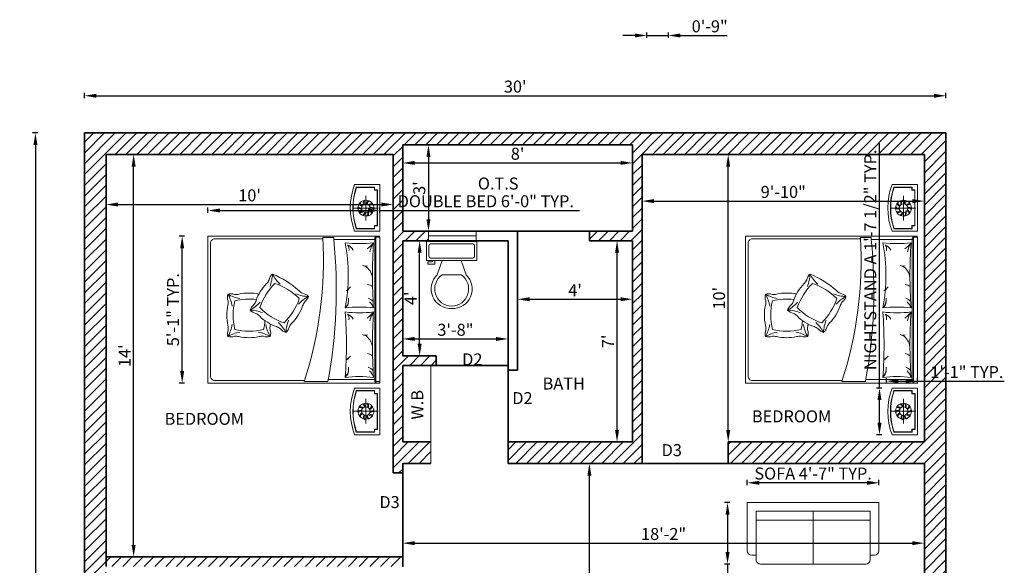
# Model space of a CAD drawing. Units: inches. Extents: x -196 to 219, y -474 to 80.
# Tile 4 of 4: x -196 to 216, y -148 to 80. Entities that reach past the tile are written whole.
import ezdxf

# ---------------------------------------------------------------- set-up
doc = ezdxf.new("R2010")
doc.units = ezdxf.units.IN
doc.header["$PDMODE"] = 35
doc.header["$PDSIZE"] = 5
for name, color, linetype, lineweight in [('A-ANNO-DIMS', 2, 'Continuous', 18), ('A-ANNO-TEXT', 7, 'Continuous', 18), ('A-AREA-IDEN', 7, 'Continuous', 25), ('A-FLOR-FIXT', 9, 'Continuous', 18), ('A-GLAZ', 4, 'Continuous', 18), ('A-WALL', 7, 'Continuous', 35), ('A-WALL-PATT', 252, 'Continuous', 13), ('furn', 28, 'Continuous', 18)]:
    doc.layers.add(name, color=color, linetype=linetype, lineweight=lineweight)
doc.styles.get("Standard").update_dxf_attribs({"font": 'arial.ttf'})
doc.dimstyles.new('ISO-25', dxfattribs={"dimtxt": 5, "dimasz": 5, "dimexe": 1.25, "dimexo": 0.625, "dimtad": 1, "dimlunit": 3, "dimtxsty": 'Standard', "dimcen": 2.5, "dimadec": 0, "dimazin": 0, "dimtfac": 1, "dimtmove": 0, "dimatfit": 3, "dimfxl": 1, "dimfxlon": 1, "dimarcsym": 0})

# ---------------------------------------------------------------- blocks, each defined once
blk = doc.blocks.new('*U3')
for p, q in [((9.5, -6), (9.5, -2)), ((-8, -8.5), (-8, -8)), ((-7, -8), (-7, -9.5)), ((-4, -8), (-6, -14)), ((4, -8), (6, -14)), ((-10, -8.5), (-8, -8.5)), ((-10, -9.5), (-10, -8.5)), ((-7, -9.5), (-10, -9.5)), ((4, -14), (-4, -14))]:
    blk.add_line(p, q)
blk.add_lwpolyline([(10.5, -8), (10.5, 0), (-10.5, 0), (-10.5, -8)], close=True)
for points in [[(-9.5, -2), (-9.5, -6)], [(8.5, -1), (-8.5, -1)], [(-8.5, -7), (8.5, -7)]]:
    blk.add_lwpolyline(points)
for centre, radius, start, end in [((-8.625, -1.875), 0.8839, 81.8699, 188.1301), ((8.625, -1.875), 0.8839, 351.8699, 98.1301), ((-8.625, -6.125), 0.8839, 171.869898, 278.1301), ((8.625, -6.125), 0.8839, 261.8699, 8.1301), ((-0.4772, -19.9188), 8.0953, 133.01722, 273.38), ((0.0374, -19.8731), 7.127, 124.50543, 269.7), ((-0.0373, -19.8731), 7.127, 270.3, 55.4946), ((0.4773, -19.9188), 8.0953, 266.62, 46.9828)]:
    blk.add_arc(centre, radius, start, end)
blk = doc.blocks.new('sofa-6')
at = {"color": 0, "linetype": 'ByBlock'}
for p, q in [((1.35, 0.7), (0.15, 0.7)), ((0.75, 0.1), (0.75, 0.7)), ((0.1, 0.6), (0.05, 0.6)), ((0.1, 0.65), (0.1, 0.1)), ((1.4, 0.1), (1.4, 0.65)), ((1.45, 0.6), (1.4, 0.6)), ((0, 0.55), (0, 0)), ((1.5, 0), (1.5, 0.55)), ((0.1, 0.2), (1.4, 0.2)), ((0, 0), (1.5, 0)), ((0.1, 0.1), (1.4, 0.1))]:
    blk.add_line(p, q, dxfattribs=at)
for centre, start, end in [((0.15, 0.65), 90, 180), ((1.35, 0.65), 360, 90), ((0.05, 0.55), 90, 180), ((1.45, 0.55), 0, 90)]:
    blk.add_arc(centre, 0.05, start, end, dxfattribs=at)
blk = doc.blocks.new('*D5')
at = {"layer": 'A-ANNO-DIMS', "color": 0, "lineweight": -2, "transparency": 16777216}
for p, q in [((-149.15, 23.91), (-146.9, 23.91)), ((-148.15, -139.09), (-148.15, 18.91)), ((-149.15, -144.09), (-146.9, -144.09))]:
    blk.add_line(p, q, dxfattribs=at)
at = {"layer": 'A-ANNO-DIMS', "color": 0, "transparency": 16777216}
for points in [[(-148.99, 18.91), (-147.32, 18.91), (-148.15, 23.91)], [(-148.99, -139.09), (-147.32, -139.09), (-148.15, -144.09)]]:
    blk.add_solid(points, dxfattribs=at)
at = {"layer": 'Defpoints', "color": 0, "transparency": 16777216}
for p in [(-159.7, 23.91), (-148.15, 23.91), (-159.7, -144.09)]:
    blk.add_point(p, dxfattribs=at)
at = {"layer": 'A-ANNO-DIMS', "color": 0, "transparency": 16777216, "insert": (-151.29, -60.09), "char_height": 5, "attachment_point": 5, "rotation": 90}
blk.add_mtext("14'", dxfattribs=at)
blk = doc.blocks.new('*D6')
at = {"layer": 'A-ANNO-DIMS', "color": 0, "lineweight": -2, "transparency": 16777216}
for p, q in [((-159.7, 4.04), (-159.7, 1.79)), ((-154.7, 3.04), (-44.7, 3.04)), ((-39.7, 4.04), (-39.7, 1.79))]:
    blk.add_line(p, q, dxfattribs=at)
at = {"layer": 'A-ANNO-DIMS', "color": 0, "transparency": 16777216}
for points in [[(-154.7, 3.87), (-154.7, 2.2), (-159.7, 3.04)], [(-44.7, 3.87), (-44.7, 2.2), (-39.7, 3.04)]]:
    blk.add_solid(points, dxfattribs=at)
at = {"layer": 'Defpoints', "color": 0, "transparency": 16777216}
for p in [(-159.7, 23.91), (-39.7, 23.91), (-39.7, 3.04)]:
    blk.add_point(p, dxfattribs=at)
at = {"layer": 'A-ANNO-DIMS', "color": 0, "transparency": 16777216, "insert": (-99.7, 6.21), "char_height": 5, "attachment_point": 5}
blk.add_mtext("10'", dxfattribs=at)
blk = doc.blocks.new('*D7')
at = {"layer": 'A-ANNO-DIMS', "color": 0, "lineweight": -2, "transparency": 16777216}
for p, q in [((-25.95, 27.91), (-23.7, 27.91)), ((-24.95, 22.91), (-24.95, -3.09)), ((-25.95, -8.09), (-23.7, -8.09))]:
    blk.add_line(p, q, dxfattribs=at)
at = {"layer": 'A-ANNO-DIMS', "color": 0, "transparency": 16777216}
for points in [[(-25.78, 22.91), (-24.12, 22.91), (-24.95, 27.91)], [(-25.78, -3.09), (-24.12, -3.09), (-24.95, -8.09)]]:
    blk.add_solid(points, dxfattribs=at)
at = {"layer": 'Defpoints', "color": 0, "transparency": 16777216}
for p in [(-35.7, 27.91), (-35.7, -8.09), (-24.95, -8.09)]:
    blk.add_point(p, dxfattribs=at)
at = {"layer": 'A-ANNO-DIMS', "color": 0, "transparency": 16777216, "insert": (-28.13, 9.91), "char_height": 5, "attachment_point": 5, "rotation": 90}
blk.add_mtext("3'", dxfattribs=at)
blk = doc.blocks.new('*D8')
at = {"layer": 'A-ANNO-DIMS', "color": 0, "lineweight": -2, "transparency": 16777216}
for p, q in [((-35.7, 21.4), (-35.7, 19.15)), ((60.3, 21.4), (60.3, 19.15)), ((-30.7, 20.4), (55.3, 20.4))]:
    blk.add_line(p, q, dxfattribs=at)
at = {"layer": 'A-ANNO-DIMS', "color": 0, "transparency": 16777216}
for points in [[(-30.7, 21.24), (-30.7, 19.57), (-35.7, 20.4)], [(55.3, 21.24), (55.3, 19.57), (60.3, 20.4)]]:
    blk.add_solid(points, dxfattribs=at)
at = {"layer": 'Defpoints', "color": 0, "transparency": 16777216}
for p in [(-35.7, 27.91), (60.3, 27.91), (60.3, 20.4)]:
    blk.add_point(p, dxfattribs=at)
at = {"layer": 'A-ANNO-DIMS', "color": 0, "transparency": 16777216, "insert": (12.3, 23.58), "char_height": 5, "attachment_point": 5}
blk.add_mtext("8'", dxfattribs=at)
blk = doc.blocks.new('*D9')
at = {"layer": 'A-ANNO-DIMS', "color": 0, "lineweight": -2, "transparency": 16777216}
for p, q in [((-35.7, -52.08), (-35.7, -54.33)), ((-30.7, -53.08), (3.3, -53.08)), ((8.3, -52.08), (8.3, -54.33))]:
    blk.add_line(p, q, dxfattribs=at)
at = {"layer": 'A-ANNO-DIMS', "color": 0, "transparency": 16777216}
for points in [[(-30.7, -52.24), (-30.7, -53.91), (-35.7, -53.08)], [(3.3, -52.24), (3.3, -53.91), (8.3, -53.08)]]:
    blk.add_solid(points, dxfattribs=at)
at = {"layer": 'Defpoints', "color": 0, "transparency": 16777216}
for p in [(-35.7, -50.11), (8.3, -50.11), (8.3, -53.08)]:
    blk.add_point(p, dxfattribs=at)
at = {"layer": 'A-ANNO-DIMS', "color": 0, "transparency": 16777216, "insert": (-13.7, -49.9), "char_height": 5, "attachment_point": 5}
blk.add_mtext('3\'-8"', dxfattribs=at)
blk = doc.blocks.new('*D10')
at = {"layer": 'A-ANNO-DIMS', "color": 0, "lineweight": -2, "transparency": 16777216}
for p, q in [((-29.64, -12.09), (-27.39, -12.09)), ((-28.64, -55.09), (-28.64, -17.09)), ((-29.64, -60.09), (-27.39, -60.09))]:
    blk.add_line(p, q, dxfattribs=at)
at = {"layer": 'A-ANNO-DIMS', "color": 0, "transparency": 16777216}
for points in [[(-29.48, -17.09), (-27.81, -17.09), (-28.64, -12.09)], [(-29.48, -55.09), (-27.81, -55.09), (-28.64, -60.09)]]:
    blk.add_solid(points, dxfattribs=at)
at = {"layer": 'Defpoints', "color": 0, "transparency": 16777216}
for p in [(-35.7, -12.09), (-28.64, -12.09), (-35.7, -60.09)]:
    blk.add_point(p, dxfattribs=at)
at = {"layer": 'A-ANNO-DIMS', "color": 0, "transparency": 16777216, "insert": (-31.77, -36.09), "char_height": 5, "attachment_point": 5, "rotation": 90}
blk.add_mtext("4'", dxfattribs=at)
blk = doc.blocks.new('*D11')
at = {"layer": 'A-ANNO-DIMS', "color": 0, "lineweight": -2, "transparency": 16777216}
for p, q in [((12.3, -37.51), (12.3, -35.26)), ((17.3, -36.51), (55.3, -36.51)), ((60.3, -37.51), (60.3, -35.26))]:
    blk.add_line(p, q, dxfattribs=at)
at = {"layer": 'A-ANNO-DIMS', "color": 0, "transparency": 16777216}
for points in [[(17.3, -35.67), (17.3, -37.34), (12.3, -36.51)], [(55.3, -35.67), (55.3, -37.34), (60.3, -36.51)]]:
    blk.add_solid(points, dxfattribs=at)
at = {"layer": 'Defpoints', "color": 0, "transparency": 16777216}
for p in [(60.3, -36.51), (12.3, -44.73), (60.3, -44.73)]:
    blk.add_point(p, dxfattribs=at)
at = {"layer": 'A-ANNO-DIMS', "color": 0, "transparency": 16777216, "insert": (36.3, -33.38), "char_height": 5, "attachment_point": 5}
blk.add_mtext("4'", dxfattribs=at)
blk = doc.blocks.new('*D12')
at = {"layer": 'A-ANNO-DIMS', "color": 0, "lineweight": -2, "transparency": 16777216}
for p, q in [((54.85, -12.09), (52.6, -12.09)), ((53.85, -91.09), (53.85, -17.09)), ((54.85, -96.09), (52.6, -96.09))]:
    blk.add_line(p, q, dxfattribs=at)
at = {"layer": 'A-ANNO-DIMS', "color": 0, "transparency": 16777216}
for points in [[(53.01, -17.09), (54.68, -17.09), (53.85, -12.09)], [(53.01, -91.09), (54.68, -91.09), (53.85, -96.09)]]:
    blk.add_solid(points, dxfattribs=at)
at = {"layer": 'Defpoints', "color": 0, "transparency": 16777216}
for p in [(53.85, -12.09), (60.3, -12.09), (60.3, -96.09)]:
    blk.add_point(p, dxfattribs=at)
at = {"layer": 'A-ANNO-DIMS', "color": 0, "transparency": 16777216, "insert": (50.72, -54.09), "char_height": 5, "attachment_point": 5, "rotation": 90}
blk.add_mtext("7'", dxfattribs=at)
blk = doc.blocks.new('*D13')
at = {"layer": 'A-ANNO-DIMS', "color": 0, "lineweight": -2, "transparency": 16777216}
for p, q in [((64.3, 5.47), (64.3, 3.22)), ((69.3, 4.47), (177.3, 4.47)), ((182.3, 5.47), (182.3, 3.22))]:
    blk.add_line(p, q, dxfattribs=at)
at = {"layer": 'A-ANNO-DIMS', "color": 0, "transparency": 16777216}
for points in [[(69.3, 5.3), (69.3, 3.63), (64.3, 4.47)], [(177.3, 5.3), (177.3, 3.63), (182.3, 4.47)]]:
    blk.add_solid(points, dxfattribs=at)
at = {"layer": 'Defpoints', "color": 0, "transparency": 16777216}
for p in [(64.3, 23.91), (182.3, 23.91), (182.3, 4.47)]:
    blk.add_point(p, dxfattribs=at)
at = {"layer": 'A-ANNO-DIMS', "color": 0, "transparency": 16777216, "insert": (123.3, 7.64), "char_height": 5, "attachment_point": 5}
blk.add_mtext('9\'-10"', dxfattribs=at)
blk = doc.blocks.new('*D14')
at = {"layer": 'A-ANNO-DIMS', "color": 0, "lineweight": -2, "transparency": 16777216}
for p, q in [((100.3, 23.91), (101.55, 23.91)), ((100.3, -91.09), (100.3, 18.91)), ((100.3, -96.09), (101.55, -96.09))]:
    blk.add_line(p, q, dxfattribs=at)
at = {"layer": 'A-ANNO-DIMS', "color": 0, "transparency": 16777216}
for points in [[(99.47, 18.91), (101.14, 18.91), (100.3, 23.91)], [(99.47, -91.09), (101.14, -91.09), (100.3, -96.09)]]:
    blk.add_solid(points, dxfattribs=at)
at = {"layer": 'Defpoints', "color": 0, "transparency": 16777216}
for p in [(100.3, 23.91), (100.3, 23.91), (100.3, -96.09)]:
    blk.add_point(p, dxfattribs=at)
at = {"layer": 'A-ANNO-DIMS', "color": 0, "transparency": 16777216, "insert": (97.12, -36.09), "char_height": 5, "attachment_point": 5, "rotation": 90}
blk.add_mtext("10'", dxfattribs=at)
blk = doc.blocks.new('*D15')
at = {"layer": 'A-ANNO-DIMS', "color": 0, "lineweight": -2, "transparency": 16777216}
for p, q in [((-35.7, -137.33), (-35.7, -139.58)), ((-30.7, -138.33), (177.3, -138.33)), ((182.3, -138.33), (182.3, -137.08))]:
    blk.add_line(p, q, dxfattribs=at)
at = {"layer": 'A-ANNO-DIMS', "color": 0, "transparency": 16777216}
for points in [[(-30.7, -137.5), (-30.7, -139.16), (-35.7, -138.33)], [(177.3, -137.5), (177.3, -139.16), (182.3, -138.33)]]:
    blk.add_solid(points, dxfattribs=at)
at = {"layer": 'Defpoints', "color": 0, "transparency": 16777216}
for p in [(-35.7, -126.59), (182.3, -138.33), (182.3, -138.33)]:
    blk.add_point(p, dxfattribs=at)
at = {"layer": 'A-ANNO-DIMS', "color": 0, "transparency": 16777216, "insert": (73.3, -135.15), "char_height": 5, "attachment_point": 5}
blk.add_mtext('18\'-2"', dxfattribs=at)
blk = doc.blocks.new('*D16')
at = {"layer": 'A-ANNO-DIMS', "color": 0, "lineweight": -2, "transparency": 16777216}
for p, q in [((43.3, -105.09), (41.05, -105.09)), ((42.3, -238.09), (42.3, -110.09)), ((43.3, -243.09), (41.05, -243.09))]:
    blk.add_line(p, q, dxfattribs=at)
at = {"layer": 'A-ANNO-DIMS', "color": 0, "transparency": 16777216}
for points in [[(41.47, -110.09), (43.14, -110.09), (42.3, -105.09)], [(41.47, -238.09), (43.14, -238.09), (42.3, -243.09)]]:
    blk.add_solid(points, dxfattribs=at)
at = {"layer": 'Defpoints', "color": 0, "transparency": 16777216}
for p in [(42.3, -105.09), (44.21, -105.09), (44.21, -243.09)]:
    blk.add_point(p, dxfattribs=at)
at = {"layer": 'A-ANNO-DIMS', "color": 0, "transparency": 16777216, "insert": (39.12, -174.09), "char_height": 5, "attachment_point": 5, "rotation": 90}
blk.add_mtext('11\'-6"', dxfattribs=at)
blk = doc.blocks.new('*D25')
at = {"layer": 'A-ANNO-DIMS', "color": 0, "lineweight": -2, "transparency": 16777216}
for p, q in [((-168.7, 47.45), (-168.7, 49.7)), ((191.3, 47.45), (191.3, 49.7)), ((-163.7, 48.45), (186.3, 48.45))]:
    blk.add_line(p, q, dxfattribs=at)
at = {"layer": 'A-ANNO-DIMS', "color": 0, "transparency": 16777216}
for points in [[(-163.7, 49.28), (-163.7, 47.61), (-168.7, 48.45)], [(186.3, 49.28), (186.3, 47.61), (191.3, 48.45)]]:
    blk.add_solid(points, dxfattribs=at)
at = {"layer": 'Defpoints', "color": 0, "transparency": 16777216}
for p in [(191.3, 48.45), (-168.7, 32.91), (191.3, 32.91)]:
    blk.add_point(p, dxfattribs=at)
at = {"layer": 'A-ANNO-DIMS', "color": 0, "transparency": 16777216, "insert": (11.3, 51.63), "char_height": 5, "attachment_point": 5}
blk.add_mtext("30'", dxfattribs=at)
blk = doc.blocks.new('*D26')
at = {"layer": 'A-ANNO-DIMS', "color": 0, "lineweight": -2, "transparency": 16777216}
for p, q in [((-188.18, 32.91), (-190.43, 32.91)), ((-189.18, 27.91), (-189.18, -394.09)), ((-188.18, -399.09), (-190.43, -399.09))]:
    blk.add_line(p, q, dxfattribs=at)
at = {"layer": 'A-ANNO-DIMS', "color": 0, "transparency": 16777216}
for points in [[(-190.01, 27.91), (-188.35, 27.91), (-189.18, 32.91)], [(-190.01, -394.09), (-188.35, -394.09), (-189.18, -399.09)]]:
    blk.add_solid(points, dxfattribs=at)
at = {"layer": 'Defpoints', "color": 0, "transparency": 16777216}
for p in [(-168.7, 32.91), (-189.18, -399.09), (-168.7, -399.09)]:
    blk.add_point(p, dxfattribs=at)
at = {"layer": 'A-ANNO-DIMS', "color": 0, "transparency": 16777216, "insert": (-192.36, -183.09), "char_height": 5, "attachment_point": 5, "rotation": 90}
blk.add_mtext("36'", dxfattribs=at)
blk = doc.blocks.new('BED-DOUBLE')
for p, q in [((70.2, 59.88), (52.52, 59.88)), ((69.67, 60.18), (69.67, 1.06)), ((70.2, 1.4), (50.22, 1.4))]:
    blk.add_line(p, q)
for points in [[(71.86, 61.24), (0, 61.24), (0, 0), (71.86, 0)], [(71.86, 0.57), (70.2, 0.57), (70.2, 60.89), (71.86, 60.89), (71.86, 0)]]:
    blk.add_lwpolyline(points)
for points in [[(48.05, 60.18), (2.83, 60.18, 0.414214), (1.06, 58.41), (1.06, 2.83, 0.414214), (2.83, 1.06), (40.4, 1.06)], [(25.84, 40.29, 0.091296), (26.93, 45.48, 0.091296), (30.19, 41.3, 0.091296)], [(27.91, 41.58, 0.111006), (21.62, 31.47, 0.119549), (31.85, 25.09, 0.107813), (38.17, 35.17)], [(38.16, 35.23, 0.121865), (27.91, 41.58, 0.121865)], [(10.11, 32.11, 0.091296), (8.3, 37.09, 0.091296), (13.27, 35.26, 0.091296)], [(36.77, 37.19, 0.091296), (41.96, 36.12, 0.091296), (37.79, 32.85, 0.091296)], [(11.19, 34.3, 0.111006), (11.2, 22.39, 0.119549), (23.25, 22.39, 0.033212), (23.81, 26.05)], [(22.76, 29.38, 0.091296), (17.57, 30.45, 0.091296), (21.75, 33.72)], [(17.57, 30.45, 0.159461), (20.01, 29.08, -0.076283), (21.52, 28, 0.115075), (28.65, 23.55, -0.076283), (30.29, 22.67, 0.159461), (32.6, 21.09)], [(33.69, 26.28, 0.091296), (32.6, 21.09, 0.091296), (29.35, 25.28, 0.091296)], [(13.27, 21.22, 0.091296), (8.3, 19.39, 0.091296), (10.11, 24.37)], [(24.18, 24.37, 0.091296), (26, 19.39, 0.091296), (21.02, 21.22, 0.091296)], [(8.3, 19.39, 0.159461), (11.08, 19.51, -0.076283), (12.94, 19.39, 0.115075), (21.35, 19.39, -0.076283), (23.21, 19.51, 0.159461), (26, 19.39)]]:
    blk.add_lwpolyline(points, format="xyb")
for points in [[(52.52, 60.71), (52.52, 59.88, -0.072944), (50.05, 0.57), (40.23, 0.57, 0.092568), (48.02, 60.71)], [(57.36, 58.53, 0.058596), (69.19, 58.53, 0.036889), (69.19, 31.42, 0.052163), (57.36, 31.42, 0.093111)], [(57.36, 29.66, 0.058596), (69.19, 29.66, 0.036648), (69.19, 2.37, 0.052163), (57.36, 2.37, 0.036967)]]:
    blk.add_lwpolyline(points, format="xyb", close=True)
for centre, radius, start, end in [((58.12, 67.4), 14.18, 306.4935, 321.2792), ((79.08, 52.23), 11.72, 147.5379, 167.5233), ((70.74, 60.18), 1.06, 90, 180), ((56.26, 55.91), 2.69, 346.4823, 38.5563), ((57.08, 53.87), 3.93, 24.2916, 70.9896), ((29.97, 42.18), 4.49, 132.6522, 168.8929), ((12.27, 9.6), 38.76, 48.3818, 67.7644), ((65.82, 51.76), 2.94, 245.8927, 286.1192), ((62.17, 43.24), 6.56, 6.6849, 58.3182), ((37.6, 28.47), 18.5, 135.1307, 161.3884), ((20.09, 45.81), 6.15, 315.7718, 333.2208), ((12.62, 35.9), 4.49, 164.5791, 200.8198), ((9.5, 32.77), 4.49, 69.3666, 105.6073), ((11.62, 43.09), 6.15, 265.0387, 282.4877), ((17.15, 19.08), 18.5, 76.8711, 103.1289), ((42.31, 42.96), 6.15, 225.5854, 243.0343), ((38.65, 33.09), 4.49, 42.4658, 78.7065), ((57.86, 39.62), 0.992, 263.7543, 347.2187), ((49.13, 50.55), 14.78, 306.2085, 315.0849), ((65.9, 36.61), 4.6, 51.8174, 79.8987), ((2.31, 33.75), 6.15, 347.6988, 5.1477), ((17.27, 9.95), 25.09, 83.1956, 104.0284), ((14.27, 36.4), 6.15, 323.2983, 340.7472), ((45.34, 30.19), 6.15, 143.2983, 160.7472), ((37.79, 37.3), 4.33, 307.2937, 344.0973), ((53.97, 34.88), 4.84, 314.406, 6.8342), ((55.66, 33.97), 3.07, 303.6349, 0.8456), ((65.25, 30.79), 4.95, 40.5354, 70.3558), ((61.08, 27.7), 8.92, 24.6457, 44.1585), ((26.34, 28.3), 18.5, 167.0576, 193.3153), ((22.41, 28.73), 5.13, 128.7754, 160.3571), ((22.01, 38.11), 18.5, 315.1307, 341.3884), ((58.12, 38.53), 14.18, 306.4935, 321.2792), ((79.08, 23.37), 11.72, 147.5379, 167.5233), ((39.53, 20.78), 6.15, 135.7718, 153.2208), ((56.26, 27.04), 2.69, 346.4823, 38.5563), ((57.08, 25), 3.93, 24.2916, 70.9896), ((13.31, 20.48), 5.13, 160.7023, 192.284), ((2.34, 22.69), 6.15, 355.2252, 12.6741), ((32.04, 22.79), 6.15, 167.6988, 185.1477), ((22.07, 20.71), 4.14, 341.3996, 21.5774), ((8.01, 28.24), 18.5, 347.0576, 348.7033), ((29.96, 24.29), 4.14, 309.4726, 349.6505), ((65.82, 22.89), 2.94, 245.8927, 286.1192), ((62.17, 14.37), 6.56, 6.6849, 58.3182), ((57.86, 10.75), 0.992, 263.7543, 347.2187), ((49.13, 21.68), 14.78, 306.2085, 315.0849), ((65.9, 7.74), 4.6, 51.8174, 79.8987), ((53.97, 6.01), 4.84, 314.406, 6.8342), ((55.66, 5.1), 3.07, 303.6349, 0.8456), ((65.25, 1.92), 4.95, 40.5354, 70.3558), ((61.08, -1.17), 8.92, 24.6457, 44.1585), ((70.74, 1.06), 1.06, 180, 270)]:
    blk.add_arc(centre, radius, start, end)
blk = doc.blocks.new('NIGHTSTAND-A')
for p, q in [((6.52, 4.73), (6.52, 14.94)), ((1.42, 9.84), (11.63, 9.84))]:
    blk.add_line(p, q)
blk.add_lwpolyline([(1.77, 0), (12.39, 0), (12.39, 19.47), (1.77, 19.47, 0.181818)], format="xyb", close=True)
for points in [[(10.16, 18.41), (2.51, 18.41, 0.167087), (2.51, 1.06), (10.16, 1.06)], [(10.16, 18.3), (2.59, 18.3, 0.165559), (2.59, 1.17), (10.16, 1.17)]]:
    blk.add_lwpolyline(points, format="xyb")
for points in [[(11.33, 17.13), (10.05, 17.13), (10.05, 18.41)], [(11.33, 17.24), (10.16, 17.24), (10.16, 18.41)], [(11.22, 2.23), (11.22, 17.24)], [(11.33, 2.23), (11.33, 17.24)], [(11.33, 2.34), (10.05, 2.34), (10.05, 1.06)], [(11.33, 2.23), (10.16, 2.23), (10.16, 1.06)]]:
    blk.add_lwpolyline(points)
for radius in [3.33, 1.81]:
    blk.add_circle((6.52, 9.84), radius)
for centre, radius, start, end in [((4.49, 11.21), 1.63, 13.462, 73.6998), ((4.33, 11.07), 2.14, 15.5103, 61.83), ((5.68, 12.14), 1.63, 337.462, 37.6998), ((5.47, 12.12), 2.14, 339.5103, 25.83), ((4.68, 8.13), 2.14, 87.5103, 133.83), ((4.59, 8.33), 1.63, 85.462, 145.6998), ((4.07, 9.75), 1.63, 49.462, 109.6998), ((4.02, 9.54), 2.14, 51.5103, 97.83), ((6.03, 7.37), 2.14, 123.5103, 169.83), ((5.85, 7.48), 1.63, 121.462, 181.6998), ((8.97, 9.92), 1.63, 229.462, 289.6998), ((7.2, 12.19), 1.63, 301.462, 1.6998), ((7.01, 12.3), 2.14, 303.5103, 349.83), ((8.37, 11.54), 2.14, 267.5103, 313.83), ((8.45, 11.35), 1.63, 265.462, 325.6998), ((7.67, 7.31), 2.14, 159.5103, 205.83), ((7.45, 7.29), 1.63, 157.462, 217.6998), ((8.81, 8.36), 2.14, 195.5103, 241.83), ((8.65, 8.22), 1.63, 193.462, 253.6998), ((9.11, 9.89), 2.14, 231.5103, 277.83)]:
    blk.add_arc(centre, radius, start, end)
blk = doc.blocks.new('NIGHTSTAND-B')
for p, q in [((6.53, 14.74), (6.53, 4.53)), ((1.42, 9.63), (11.63, 9.63))]:
    blk.add_line(p, q)
blk.add_lwpolyline([(1.77, 19.47), (12.39, 19.47), (12.39, 0), (1.77, 0, -0.181818)], format="xyb", close=True)
for points in [[(10.16, 1.06), (2.51, 1.06, -0.167087), (2.51, 18.41), (10.16, 18.41)], [(10.16, 1.17), (2.59, 1.17, -0.165559), (2.59, 18.3), (10.16, 18.3)]]:
    blk.add_lwpolyline(points, format="xyb")
for points in [[(11.33, 17.13), (10.05, 17.13), (10.05, 18.41)], [(11.33, 17.24), (10.16, 17.24), (10.16, 18.41)], [(11.22, 17.24), (11.22, 2.23)], [(11.33, 17.24), (11.33, 2.23)], [(11.33, 2.34), (10.05, 2.34), (10.05, 1.06)], [(11.33, 2.23), (10.16, 2.23), (10.16, 1.06)]]:
    blk.add_lwpolyline(points)
for radius in [3.33, 1.81]:
    blk.add_circle((6.53, 9.63), radius)
for centre, radius, start, end in [((7.58, 11.92), 2.14, 154.17, 200.4897), ((7.37, 11.94), 1.63, 142.3002, 202.538), ((8.72, 10.86), 2.14, 118.17, 164.4897), ((8.56, 11), 1.63, 106.3002, 166.538), ((4.68, 11.34), 2.14, 226.17, 272.4897), ((4.6, 11.14), 1.63, 214.3002, 274.538), ((4.08, 9.72), 1.63, 250.3002, 310.538), ((4.03, 9.93), 2.14, 262.17, 308.4897), ((6.04, 12.1), 2.14, 190.17, 236.4897), ((5.85, 11.99), 1.63, 178.3002, 238.538), ((9.03, 9.34), 2.14, 82.17, 128.4897), ((8.98, 9.55), 1.63, 70.3002, 130.538), ((7.2, 7.28), 1.63, 358.3002, 58.538), ((7.02, 7.17), 2.14, 10.17, 56.4897), ((8.37, 7.93), 2.14, 46.17, 92.4897), ((8.46, 8.12), 1.63, 34.3002, 94.538), ((4.49, 8.26), 1.63, 286.3002, 346.538), ((4.33, 8.4), 2.14, 298.17, 344.4897), ((5.69, 7.33), 1.63, 322.3002, 22.538), ((5.47, 7.35), 2.14, 334.17, 20.4897)]:
    blk.add_arc(centre, radius, start, end)
blk = doc.blocks.new('*D38')
at = {"layer": 'A-ANNO-DIMS', "color": 0, "lineweight": -2, "transparency": 16777216}
for p, q in [((-117.08, -0.45), (-117.08, 1.8)), ((-112.08, 0.55), (-50.22, 0.55)), ((-45.22, -0.45), (-45.22, 1.8)), ((-45.22, 0.55), (38.22, 0.55))]:
    blk.add_line(p, q, dxfattribs=at)
at = {"layer": 'A-ANNO-DIMS', "color": 0, "transparency": 16777216}
for points in [[(-112.08, 1.38), (-112.08, -0.29), (-117.08, 0.55)], [(-50.22, 1.38), (-50.22, -0.29), (-45.22, 0.55)]]:
    blk.add_solid(points, dxfattribs=at)
at = {"layer": 'Defpoints', "color": 0, "transparency": 16777216}
for p in [(-45.22, 0.55), (-117.08, -10.23), (-45.22, -10.23)]:
    blk.add_point(p, dxfattribs=at)
at = {"layer": 'A-ANNO-DIMS', "color": 0, "transparency": 16777216, "insert": (-1, 3.76), "char_height": 5, "attachment_point": 5}
blk.add_mtext('DOUBLE BED 6\'-0" TYP.', dxfattribs=at)
blk = doc.blocks.new('*D39')
at = {"layer": 'A-ANNO-DIMS', "color": 0, "lineweight": -2, "transparency": 16777216}
for p, q in [((-126.86, -10.23), (-129.11, -10.23)), ((-127.86, -66.47), (-127.86, -15.23)), ((-126.86, -71.47), (-129.11, -71.47))]:
    blk.add_line(p, q, dxfattribs=at)
at = {"layer": 'A-ANNO-DIMS', "color": 0, "transparency": 16777216}
for points in [[(-128.7, -15.23), (-127.03, -15.23), (-127.86, -10.23)], [(-128.7, -66.47), (-127.03, -66.47), (-127.86, -71.47)]]:
    blk.add_solid(points, dxfattribs=at)
at = {"layer": 'Defpoints', "color": 0, "transparency": 16777216}
for p in [(-127.86, -10.23), (-117.08, -10.23), (-117.08, -71.47)]:
    blk.add_point(p, dxfattribs=at)
at = {"layer": 'A-ANNO-DIMS', "color": 0, "transparency": 16777216, "insert": (-131.04, -40.85), "char_height": 5, "attachment_point": 5, "rotation": 90}
blk.add_mtext('5\'-1" TYP.', dxfattribs=at)
blk = doc.blocks.new('*D40')
at = {"layer": 'A-ANNO-DIMS', "color": 0, "lineweight": -2, "transparency": 16777216}
for p, q in [((163.52, -73.6), (163.52, 28.48)), ((164.52, -73.6), (162.27, -73.6)), ((163.52, -88.07), (163.52, -78.6)), ((164.52, -93.07), (162.27, -93.07))]:
    blk.add_line(p, q, dxfattribs=at)
at = {"layer": 'A-ANNO-DIMS', "color": 0, "transparency": 16777216}
for points in [[(162.68, -78.6), (164.35, -78.6), (163.52, -73.6)], [(162.68, -88.07), (164.35, -88.07), (163.52, -93.07)]]:
    blk.add_solid(points, dxfattribs=at)
at = {"layer": 'Defpoints', "color": 0, "transparency": 16777216}
for p in [(163.52, -73.6), (166.44, -73.6), (166.44, -93.07)]:
    blk.add_point(p, dxfattribs=at)
at = {"layer": 'A-ANNO-DIMS', "color": 0, "transparency": 16777216, "insert": (160.31, -20.06), "char_height": 5, "attachment_point": 5, "rotation": 90}
blk.add_mtext('NIGHTSTAND A 1\'-7 1/2" TYP.', dxfattribs=at)
blk = doc.blocks.new('*D41')
at = {"layer": 'A-ANNO-DIMS', "color": 0, "lineweight": -2, "transparency": 16777216}
for p, q in [((166.44, -71.68), (166.44, -69.43)), ((179.42, -71.68), (179.42, -69.43)), ((171.44, -70.68), (174.42, -70.68)), ((179.42, -70.68), (215.67, -70.68))]:
    blk.add_line(p, q, dxfattribs=at)
at = {"layer": 'A-ANNO-DIMS', "color": 0, "transparency": 16777216}
for points in [[(171.44, -69.84), (171.44, -71.51), (166.44, -70.68)], [(174.42, -69.84), (174.42, -71.51), (179.42, -70.68)]]:
    blk.add_solid(points, dxfattribs=at)
at = {"layer": 'Defpoints', "color": 0, "transparency": 16777216}
for p in [(166.44, -73.6), (179.42, -70.68), (179.42, -73.6)]:
    blk.add_point(p, dxfattribs=at)
at = {"layer": 'A-ANNO-DIMS', "color": 0, "transparency": 16777216, "insert": (200.04, -67.54), "char_height": 5, "attachment_point": 5}
blk.add_mtext('1\'-1" TYP.', dxfattribs=at)
blk = doc.blocks.new('*D44')
at = {"layer": 'A-ANNO-DIMS', "color": 0, "lineweight": -2, "transparency": 16777216}
for p, q in [((108.28, -114.12), (108.28, -111.87)), ((158.27, -113.12), (113.28, -113.12)), ((163.27, -114.12), (163.27, -111.87))]:
    blk.add_line(p, q, dxfattribs=at)
at = {"layer": 'A-ANNO-DIMS', "color": 0, "transparency": 16777216}
for points in [[(113.28, -112.29), (113.28, -113.96), (108.28, -113.12)], [(158.27, -112.29), (158.27, -113.96), (163.27, -113.12)]]:
    blk.add_solid(points, dxfattribs=at)
at = {"layer": 'Defpoints', "color": 0, "transparency": 16777216}
for p in [(108.28, -113.12), (108.28, -121.37), (163.27, -121.37)]:
    blk.add_point(p, dxfattribs=at)
at = {"layer": 'A-ANNO-DIMS', "color": 0, "transparency": 16777216, "insert": (135.77, -109.91), "char_height": 5, "attachment_point": 5}
blk.add_mtext('SOFA 4\'-7" TYP.', dxfattribs=at)
blk = doc.blocks.new('*D45')
at = {"layer": 'A-ANNO-DIMS', "color": 0, "lineweight": -2, "transparency": 16777216}
for p, q in [((101.03, -121.37), (98.78, -121.37)), ((100.03, -126.37), (100.03, -142.04)), ((101.03, -147.04), (98.78, -147.04)), ((100.03, -147.04), (100.03, -195.5))]:
    blk.add_line(p, q, dxfattribs=at)
at = {"layer": 'A-ANNO-DIMS', "color": 0, "transparency": 16777216}
for points in [[(99.19, -126.37), (100.86, -126.37), (100.03, -121.37)], [(99.19, -142.04), (100.86, -142.04), (100.03, -147.04)]]:
    blk.add_solid(points, dxfattribs=at)
at = {"layer": 'Defpoints', "color": 0, "transparency": 16777216}
for p in [(108.28, -121.37), (100.03, -147.04), (108.28, -147.04)]:
    blk.add_point(p, dxfattribs=at)
at = {"layer": 'A-ANNO-DIMS', "color": 0, "transparency": 16777216, "insert": (96.82, -173.77), "char_height": 5, "attachment_point": 5, "rotation": 90}
blk.add_mtext('2\'-1 1/2" TYP.', dxfattribs=at)
blk = doc.blocks.new('*D58')
at = {"layer": 'A-ANNO-DIMS', "color": 0, "lineweight": -2, "transparency": 16777216}
for p, q in [((-21.7, -454.04), (-21.7, -456.29)), ((-16.7, -455.04), (3.3, -455.04)), ((8.3, -454.04), (8.3, -456.29))]:
    blk.add_line(p, q, dxfattribs=at)
at = {"layer": 'A-ANNO-DIMS', "color": 0, "transparency": 16777216}
for points in [[(-16.7, -454.21), (-16.7, -455.88), (-21.7, -455.04)], [(3.3, -454.21), (3.3, -455.88), (8.3, -455.04)]]:
    blk.add_solid(points, dxfattribs=at)
at = {"layer": 'Defpoints', "color": 0, "transparency": 16777216}
for p in [(-21.7, -60.09), (8.3, -64.09), (8.3, -455.04)]:
    blk.add_point(p, dxfattribs=at)
at = {"layer": 'A-ANNO-DIMS', "color": 0, "transparency": 16777216, "insert": (-6.7, -451.87), "char_height": 5, "attachment_point": 5}
blk.add_mtext('2\'-6"', dxfattribs=at)
blk = doc.blocks.new('*D60')
at = {"layer": 'A-ANNO-DIMS', "color": 0, "lineweight": -2, "transparency": 16777216}
for p, q in [((66.3, 72.61), (66.3, 74.86)), ((75.3, 72.61), (75.3, 74.86)), ((61.3, 73.61), (56.3, 73.61)), ((66.3, 73.61), (75.3, 73.61)), ((80.3, 73.61), (99.84, 73.61))]:
    blk.add_line(p, q, dxfattribs=at)
at = {"layer": 'A-ANNO-DIMS', "color": 0, "transparency": 16777216}
for points in [[(61.3, 74.45), (61.3, 72.78), (66.3, 73.61)], [(80.3, 74.45), (80.3, 72.78), (75.3, 73.61)]]:
    blk.add_solid(points, dxfattribs=at)
at = {"layer": 'Defpoints', "color": 0, "transparency": 16777216}
for p in [(75.3, 73.61), (66.3, -339.09), (75.3, -348.09)]:
    blk.add_point(p, dxfattribs=at)
at = {"layer": 'A-ANNO-DIMS', "color": 0, "transparency": 16777216, "insert": (92.57, 76.79), "char_height": 5, "attachment_point": 5}
blk.add_mtext('0\'-9"', dxfattribs=at)

msp = doc.modelspace()

# ---------------------------------------------------------------- hatches: boundary and pattern name
at = {"layer": 'A-WALL-PATT'}
h = msp.add_hatch(dxfattribs=at)
h.set_pattern_fill('ANSI31', color=256)
h.set_pattern_definition([(45, (-560.5042, 72.7454), (-2.245064, 2.245064), [])])
h.paths.add_polyline_path([(-159.698, -243.094), (-159.698, -148.094), (-159.698, 23.906), (-39.698, 23.906), (-39.698, -108.969), (-35.698, -108.969), (-35.698, -105.094), (-23.894, -105.094), (-23.894, -96.094), (-35.698, -96.094), (-35.698, -64.094), (-21.698, -64.094), (-21.698, -60.094), (-35.698, -60.094), (-35.698, -12.094), (-24.951, -12.094), (-24.951, -8.094), (-35.698, -8.094), (-35.698, 23.906), (-35.698, 27.906), (60.302, 27.906), (60.302, 23.906), (60.302, -8.094), (42.302, -8.094), (42.302, -12.094), (60.302, -12.094), (60.302, -96.094), (42.302, -96.094), (8.302, -96.094), (8.302, -105.094), (42.302, -105.094), (60.302, -105.094), (64.302, -105.094), (64.302, 23.906), (182.302, 23.906), (182.302, -96.094), (100.302, -96.094), (100.302, -105.094), (182.302, -105.094), (182.302, -252.094), (191.302, -252.094), (191.302, 32.906), (-168.698, 32.906), (-168.698, -399.094), (-134.786, -399.094), (-134.786, -390.094), (-159.698, -390.094)])
h.paths.add_polyline_path([(191.302, -252.094), (187.302, -252.094), (187.302, -420.094), (183.555, -420.094), (183.555, -429.094), (191.302, -429.094)])
h.paths.add_polyline_path([(87.555, -420.094), (75.302, -420.094), (38.543, -420.094), (3.06, -420.094), (3.06, -425.094), (3.06, -429.094), (87.555, -429.094)])
h.paths.add_polyline_path([(75.302, -252.094), (81.302, -252.094), (81.302, -243.094), (0.302, -243.094), (0.302, -252.094), (66.302, -252.094), (66.302, -339.094), (37.784, -339.094), (37.784, -348.094), (66.302, -348.094), (75.302, -348.094)], flags=17)
h.paths.add_polyline_path([(-16.216, -339.094), (-35.698, -339.094), (-35.698, -243.094), (-43.698, -243.094), (-43.698, -252.094), (-39.698, -252.094), (-39.698, -352.094), (-35.698, -352.094), (-35.698, -348.094), (-16.216, -348.094)], flags=17)
h.paths.add_polyline_path([(-79.698, -243.094), (-159.698, -243.094), (-159.698, -252.094), (-79.698, -252.094)], flags=17)
h.paths.add_polyline_path([(-35.698, -144.094), (-159.698, -144.094), (-159.698, -148.094), (-35.698, -148.094)], flags=17)

# ---------------------------------------------------------------- linework, layer by layer
at = {"layer": 'A-FLOR-FIXT'}
msp.add_line((-23.894, -64.094), (-23.894, -105.094), dxfattribs=at)
at = {"layer": 'A-GLAZ'}
for p, q in [((-24.951, -8.094), (-24.951, -12.094)), ((-4.951, -8.094), (-4.951, -12.094)), ((-24.951, -10.094), (-4.951, -10.094))]:
    msp.add_line(p, q, dxfattribs=at)
at = {"layer": 'A-WALL'}
for p, q in [((-168.698, 32.906), (191.302, 32.906)), ((-168.698, -399.094), (-168.698, 32.906)), ((191.302, 32.906), (191.302, -252.094)), ((-35.698, 27.906), (60.302, 27.906)), ((-35.698, 23.906), (-35.698, 27.906)), ((60.302, 23.906), (60.302, 27.906)), ((-159.698, 23.906), (-39.698, 23.906)), ((-159.698, -148.094), (-159.698, 23.906)), ((-39.698, -108.969), (-39.698, 23.906)), ((-35.698, -8.094), (-35.698, 23.906)), ((60.302, -8.094), (60.302, 23.906)), ((64.302, -105.094), (64.302, 23.906)), ((64.302, 23.906), (182.302, 23.906)), ((182.302, 23.906), (182.302, -96.094)), ((60.302, -8.094), (-35.698, -8.094)), ((12.302, -12.094), (12.302, -8.094)), ((42.302, -8.094), (42.302, -12.094)), ((8.302, -12.094), (-35.698, -12.094)), ((-35.698, -60.094), (-35.698, -12.094)), ((8.302, -105.094), (8.302, -12.094)), ((12.302, -66.094), (12.302, -12.094)), ((60.302, -12.094), (42.302, -12.094)), ((60.302, -96.094), (60.302, -12.094)), ((-21.698, -60.094), (-35.698, -60.094)), ((-21.698, -64.094), (-21.698, -60.094)), ((8.302, -64.094), (-35.698, -64.094)), ((-35.698, -96.094), (-35.698, -64.094)), ((12.302, -66.094), (8.302, -66.094)), ((-23.894, -96.094), (-35.698, -96.094)), ((42.302, -96.094), (8.302, -96.094)), ((60.302, -96.094), (42.302, -96.094)), ((100.302, -96.094), (182.302, -96.094)), ((100.302, -96.094), (100.302, -105.094)), ((-23.894, -105.094), (-35.698, -105.094)), ((-35.698, -148.094), (-35.698, -105.094)), ((42.302, -105.094), (8.302, -105.094)), ((60.302, -105.094), (42.302, -105.094)), ((60.302, -105.094), (64.302, -105.094)), ((64.302, -105.094), (182.302, -105.094)), ((182.302, -105.094), (182.302, -252.094)), ((-35.698, -108.969), (-39.698, -108.969)), ((-159.698, -144.094), (-35.698, -144.094))]:
    msp.add_line(p, q, dxfattribs=at)

# ---------------------------------------------------------------- block references
at = {"layer": 'A-FLOR-FIXT'}
msp.add_blockref('*U3', (-15.248, -12.338), dxfattribs=at)
at = {"layer": 'furn'}
for name, p in [('NIGHTSTAND-B', (-57.618, -8.108)), ('NIGHTSTAND-B', (167.022, -8.108)), ('BED-DOUBLE', (-117.084, -71.473)), ('BED-DOUBLE', (107.556, -71.473)), ('NIGHTSTAND-A', (-57.614, -93.067)), ('NIGHTSTAND-A', (167.026, -93.067))]:
    msp.add_blockref(name, p, dxfattribs=at)
at = {"layer": 'furn', "xscale": 36.66436083614781, "yscale": 36.66436083614781, "zscale": 36.66436083614781, "rotation": 180}
msp.add_blockref('sofa-6', (163.273, -121.371), dxfattribs=at)

# ---------------------------------------------------------------- texts
at = {"layer": 'A-ANNO-TEXT', "char_height": 5, "attachment_point": 1}
for s, width, insert in [('D2', 10.24911, (-10.878, -59.099)), ('D2', 4.52052, (10.079, -75.28)), ('D3', 16.30459, (72.482, -96.993)), ('D3', 9.76234, (-45.46, -118.677))]:
    msp.add_mtext_dynamic_manual_height_columns(s, width=width, gutter_width=12.5, heights=[0], dxfattribs=dict(at, insert=insert))
at = {"layer": 'A-ANNO-TEXT', "insert": (-32.125, -86.75), "char_height": 5, "attachment_point": 1, "rotation": 90}
msp.add_mtext_dynamic_manual_height_columns('W.B', width=14.9939, gutter_width=12.5, heights=[0], dxfattribs=at)
at = {"layer": 'A-AREA-IDEN', "char_height": 5, "attachment_point": 1}
for s, width, insert in [('O.T.S', 35.05382, (-4.318, 14.306)), ('BATH', 22.6998, (22.741, -69.184)), ('BEDROOM', 58.82118, (-135.23, -83.928)), ('BEDROOM', 48.86698, (110.197, -82.884))]:
    msp.add_mtext_dynamic_manual_height_columns(s, width=width, gutter_width=12.5, heights=[0], dxfattribs=dict(at, insert=insert))

# ---------------------------------------------------------------- dimensions: what is measured, and where the dimension line sits
at = {"layer": 'A-ANNO-DIMS'}
for base, p1, p2, override, picture, middle in [((75.302, 73.612), (66.302, -339.094), (75.302, -348.094), {"dimdec": 1, "dimlfac": 1, "dimrnd": 0, "dimzin": 1, "dimdsep": 46, "dimlunit": 4, "dimfrac": 2}, '*D60', (92.573, 76.79)), ((191.302, 48.447), (-168.698, 32.906), (191.302, 32.906), {"dimclrd": 0, "dimclre": 0, "dimclrt": 0}, '*D25', (11.302, 51.627)), ((60.302, 20.405), (-35.698, 27.906), (60.302, 27.906), {"dimclrd": 0, "dimclre": 0, "dimclrt": 0}, '*D8', (12.302, 23.582)), ((-39.698, 3.036), (-159.698, 23.906), (-39.698, 23.906), {"dimclrd": 0, "dimclre": 0, "dimclrt": 0}, '*D6', (-99.698, 6.214)), ((182.302, 4.465), (64.302, 23.906), (182.302, 23.906), {"dimclrd": 0, "dimclre": 0, "dimclrt": 0}, '*D13', (123.302, 7.643)), ((60.302, -36.506), (12.302, -44.733), (60.302, -44.733), {"dimclrd": 0, "dimclre": 0, "dimclrt": 0}, '*D11', (36.302, -33.381)), ((8.302, -53.076), (-35.698, -50.108), (8.302, -50.108), {"dimclrd": 0, "dimclre": 0, "dimclrt": 0}, '*D9', (-13.698, -49.897)), ((8.302, -455.044), (-21.698, -60.094), (8.302, -64.094), {"dimdec": 1, "dimlfac": 1, "dimrnd": 0, "dimzin": 1, "dimdsep": 46, "dimlunit": 4, "dimfrac": 2}, '*D58', (-6.698, -451.866)), ((182.302, -138.328), (-35.698, -126.594), (182.302, -138.328), {"dimclrd": 0, "dimclre": 0, "dimclrt": 0}, '*D15', (73.302, -135.151))]:
    dim = msp.add_linear_dim(base=base, p1=p1, p2=p2, dimstyle='ISO-25', override=override, dxfattribs=at)
    dim.commit()
    dim.dimension.update_dxf_attribs({"geometry": picture, "text_midpoint": middle})
for base, p1, p2, picture, middle in [((-189.179, -399.094), (-168.698, 32.906), (-168.698, -399.094), '*D26', (-192.358, -183.094)), ((-24.951, -8.094), (-35.698, 27.906), (-35.698, -8.094), '*D7', (-28.131, 9.906)), ((-148.153, 23.906), (-159.698, -144.094), (-159.698, 23.906), '*D5', (-151.288, -60.094)), ((100.302, 23.906), (100.302, -96.094), (100.302, 23.906), '*D14', (97.124, -36.094)), ((-28.645, -12.094), (-35.698, -60.094), (-35.698, -12.094), '*D10', (-31.77, -36.094)), ((53.848, -12.094), (60.302, -96.094), (60.302, -12.094), '*D12', (50.723, -54.094)), ((42.302, -105.094), (44.205, -243.094), (44.205, -105.094), '*D16', (39.124, -174.094))]:
    dim = msp.add_linear_dim(base=base, p1=p1, p2=p2, angle=90, dimstyle='ISO-25', override={"dimclrd": 0, "dimclre": 0, "dimclrt": 0}, dxfattribs=at)
    dim.commit()
    dim.dimension.update_dxf_attribs({"geometry": picture, "text_midpoint": middle})
for base, p1, p2, angle, text, picture, middle in [((163.516, -73.597), (166.436, -93.067), (166.436, -73.597), 90, 'NIGHTSTAND A <> TYP.', '*D40', (160.306, -20.058)), ((-127.862, -10.232), (-117.083, -71.473), (-117.083, -10.232), 90, '<> TYP.', '*D39', (-131.04, -40.853)), ((108.276, -113.122), (163.273, -121.371), (108.276, -121.371), 180, 'SOFA <> TYP.', '*D44', (135.775, -109.91)), ((100.027, -147.037), (108.276, -121.371), (108.276, -147.037), 270, '<> TYP.', '*D45', (96.817, -173.768))]:
    dim = msp.add_linear_dim(base=base, p1=p1, p2=p2, angle=angle, text=text, dimstyle='ISO-25', override={"dimdec": 1, "dimlfac": 1, "dimrnd": 0, "dimzin": 1, "dimdsep": 46, "dimlunit": 4, "dimfrac": 2}, dxfattribs=at)
    dim.commit()
    dim.dimension.update_dxf_attribs({"geometry": picture, "text_midpoint": middle})
for base, p1, p2, text, picture, middle in [((-45.223, 0.547), (-117.083, -10.232), (-45.223, -10.232), 'DOUBLE BED <> TYP.', '*D38', (-1, 3.759)), ((179.416, -70.677), (166.436, -73.597), (179.416, -73.597), '<> TYP.', '*D41', (200.044, -67.54))]:
    dim = msp.add_linear_dim(base=base, p1=p1, p2=p2, text=text, dimstyle='ISO-25', override={"dimdec": 1, "dimlfac": 1, "dimrnd": 0, "dimzin": 1, "dimdsep": 46, "dimlunit": 4, "dimfrac": 2}, dxfattribs=at)
    dim.commit()
    dim.dimension.update_dxf_attribs({"geometry": picture, "text_midpoint": middle})

doc.saveas('drawing.dxf')
